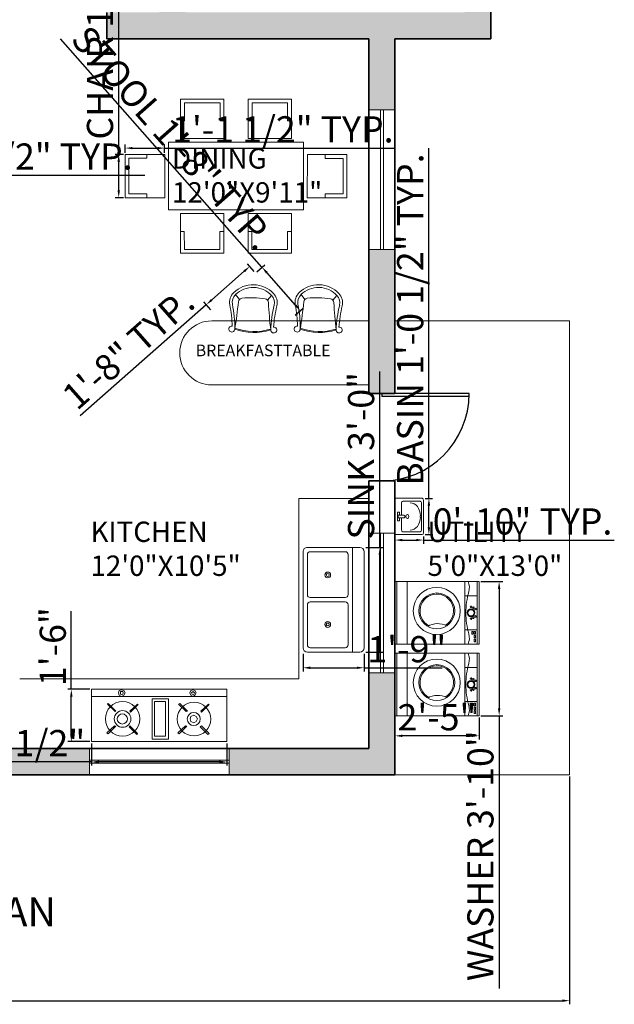
# Model space of a CAD drawing. Units: inches. Extents: x 4606 to 5879, y 1332 to 2209.
# Tile 2 of 7: x 4974 to 5178, y 1332 to 1671. Entities that reach past the tile are written whole.
import ezdxf

# ---------------------------------------------------------------- set-up
doc = ezdxf.new("R2010")
doc.units = ezdxf.units.IN
for name, color, linetype, lineweight in [('A-ANNO-DIMS', 2, 'Continuous', 18), ('A-ANNO-TEXT', 7, 'Continuous', 18), ('A-ANNO-TITL', 7, 'Continuous', 25), ('A-AREA-IDEN', 7, 'Continuous', 18), ('A-DOOR', 4, 'Continuous', 25), ('A-EQPM', 9, 'Continuous', 18), ('A-FLOR-CASE', 32, 'Continuous', 18), ('A-FLOR-PERI', 7, 'Continuous', 20), ('A-FURN', 8, 'Continuous', 18), ('A-WALL', 7, 'Continuous', 35), ('A-WALL-PATT', 252, 'Continuous', 13), ('window', 130, 'Continuous', 18), ('Сантехника', 9, 'Continuous', 18)]:
    doc.layers.add(name, color=color, linetype=linetype, lineweight=lineweight)
doc.styles.get("Standard").update_dxf_attribs({"font": 'arial.ttf'})
doc.dimstyles.new('ISO-25', dxfattribs={"dimtxt": 9, "dimasz": 2.5, "dimexe": 1.25, "dimexo": 0.625, "dimtad": 1, "dimlunit": 3, "dimtxsty": 'Standard', "dimcen": 2.5, "dimadec": 0, "dimazin": 0, "dimtfac": 1, "dimtmove": 0, "dimatfit": 3, "dimfxl": 1, "dimarcsym": 0})

# ---------------------------------------------------------------- blocks, each defined once
blk = doc.blocks.new('D2')
for p, q in [((0, 30), (0, 0)), ((1, 30), (1, 0)), ((0, 0), (1, 0))]:
    blk.add_line(p, q)
blk.add_arc((0, 0), 30, 0, 90)
blk = doc.blocks.new('A$C16EC238A')
for p, q in [((490, 810), (485, 914)), ((148, 493), (45, 507))]:
    blk.add_line(p, q)
for centre, radius, start, end in [((464, 496), 464, 87.0599, 178.502), ((464, 496), 419, 87.0599, 178.502), ((476, 730), 184, 31.9256, 87.0599), ((476, 730), 229, 31.9256, 87.0599), ((2169, 1687), 1760, 209.219, 222.7724), ((2169, 1687), 1715, 209.219, 221.1077), ((1301, -402), 1474, 132.9725, 140.5328), ((1209, -303), 1339, 124.646, 132.9725), ((486, 744), 66, 46.736, 125.0291), ((4628, 5145), 5977, 226.736, 231.1302), ((229, 502), 229, 178.502, 233.6363), ((229, 502), 184, 178.502, 233.6363), ((214, 493), 66, 140.5328, 218.8259), ((62, 930), 910, 293.6787, 331.8832), ((913, 525), 50, 222.7809, 137.6785), ((-856, -1112), 1760, 42.7895, 56.3429), ((-4494, -3296), 5977, 34.4317, 38.8259), ((62, 930), 925, 293.8563, 331.7056), ((-856, -1112), 1715, 44.4541, 56.3429), ((399, 50), 50, 127.8834, 42.7809)]:
    blk.add_arc(centre, radius, start, end)
blk = doc.blocks.new('Sink-double - 36 in top')
for p, q in [((-18, -4), (18, -4)), ((-0.75, -18.5), (-0.75, -6.5)), ((0.75, -6.5), (0.75, -18.5))]:
    blk.add_line(p, q)
for points in [[(-16.5, 0), (16.5, 0)], [(-18, -19.5), (-18, -1.5)], [(18, -1.5), (18, -19.5)], [(-16.5, -18.5), (-16.5, -6.5)], [(-15.5, -5.5), (-1.75, -5.5)], [(1.75, -5.5), (15.5, -5.5)], [(16.5, -6.5), (16.5, -18.5)], [(-1.75, -19.5), (-15.5, -19.5)], [(15.5, -19.5), (1.75, -19.5)], [(16.5, -21), (-16.5, -21)]]:
    blk.add_lwpolyline(points)
for centre, radius in [((-8.5, -12.5), 1), ((-8.5, -12.5), 0.5), ((8.5, -12.5), 1), ((8.5, -12.5), 0.5)]:
    blk.add_circle(centre, radius)
for centre, radius, start, end in [((-16.5, -1.5), 1.5, 90, 180), ((16.5, -1.5), 1.5, 0, 90), ((-15.5, -6.5), 1, 90, 180), ((-1.75, -6.5), 1, 0, 90), ((1.75, -6.5), 1, 90, 180), ((15.5, -6.5), 1, 0, 90), ((-16.5, -19.5), 1.5, 180, 270), ((-15.5, -18.5), 1, 180, 270), ((-1.75, -18.5), 1, 270, 0), ((1.75, -18.5), 1, 180, 270), ((15.5, -18.5), 1, 270, 0), ((16.5, -19.5), 1.5, 270, 0)]:
    blk.add_arc(centre, radius, start, end)
blk = doc.blocks.new('gas 1')
for points in [[(35.93, -1.87), (35.93, 0), (0, 0), (0, -1.87)], [(8.12, -0.94), (8.44, -1.56), (8.91, -1.87), (9.53, -1.56), (9.84, -0.94), (9.53, -0.31), (8.91, -0.16), (8.44, -0.31)], [(8.59, -0.94), (8.75, -1.25), (8.91, -1.41), (9.22, -1.25), (9.37, -0.94), (9.22, -0.78), (8.91, -0.62), (8.75, -0.78)], [(19.84, -13.28), (15.47, -13.28), (15.47, -2.5), (19.84, -2.5)], [(27.03, -0.94), (27.34, -1.56), (27.97, -1.87), (28.59, -1.56), (28.75, -0.94), (28.59, -0.31), (27.97, -0.16), (27.34, -0.31)], [(27.5, -0.94), (27.65, -1.25), (27.97, -1.41), (28.28, -1.25), (28.28, -0.94), (28.28, -0.62), (27.97, -0.62), (27.65, -0.62)], [(4.84, -3.91), (4.69, -4.06), (6.72, -6.09), (6.87, -5.78)], [(12.81, -3.91), (12.5, -3.75), (10.47, -5.78), (10.78, -5.94)], [(19.22, -12.5), (16.25, -12.5), (16.25, -3.28), (19.22, -3.28)], [(23.75, -3.91), (23.59, -4.06), (25.62, -6.09), (25.78, -5.78)], [(31.71, -3.91), (31.56, -3.75), (29.53, -5.78), (29.68, -5.94)], [(7.81, -7.81), (8.12, -8.59), (8.75, -8.91), (9.53, -8.59), (9.69, -7.81), (9.53, -7.19), (8.75, -6.87), (8.12, -7.19)], [(7.03, -10), (6.72, -9.69), (4.69, -11.72), (5, -12.03)], [(12.97, -11.56), (10.94, -9.69), (10.62, -9.84), (12.65, -11.87)], [(23.75, -11.72), (23.9, -12.03), (25.93, -10), (25.78, -9.69)], [(31.87, -11.56), (29.84, -9.69), (29.53, -9.84), (31.56, -11.87)]]:
    blk.add_lwpolyline(points, close=True)
blk.add_lwpolyline([(35.93, -1.87), (35.93, -13.9), (0, -13.9), (0, -1.87)])
for centre, radius in [((8.7, -7.92), 4.48), ((27.7, -7.86), 4.58), ((8.77, -7.89), 1.74), ((27.69, -7.89), 2.22), ((27.76, -7.89), 1.35)]:
    blk.add_circle(centre, radius)
blk = doc.blocks.new('wash')
at = {"layer": 'Сантехника'}
for p, q in [((4817.13, 2840.92), (4788.24, 2840.92)), ((4788.24, 2819.46), (4788.24, 2840.92)), ((4788.93, 2819.46), (4788.93, 2840.92)), ((4793.08, 2819.46), (4793.08, 2840.92)), ((4812.98, 2819.46), (4812.98, 2840.92)), ((4816.44, 2819.46), (4816.44, 2840.92)), ((4817.13, 2819.46), (4817.13, 2840.92)), ((4793.08, 2836.07), (4788.93, 2836.07)), ((4793.08, 2824.31), (4788.93, 2824.31)), ((4817.13, 2819.46), (4788.24, 2819.46)), ((4817.13, 2816.27), (4788.24, 2816.27)), ((4788.24, 2794.82), (4788.24, 2816.27)), ((4788.93, 2794.82), (4788.93, 2816.27)), ((4793.08, 2794.82), (4793.08, 2816.27)), ((4812.98, 2794.82), (4812.98, 2816.27)), ((4816.44, 2794.82), (4816.44, 2816.27)), ((4817.13, 2794.82), (4817.13, 2816.27)), ((4793.08, 2811.43), (4788.93, 2811.43)), ((4793.08, 2799.66), (4788.93, 2799.66)), ((4817.13, 2794.82), (4788.24, 2794.82))]:
    blk.add_line(p, q, dxfattribs=at)
for points in [[(4789.4, 2839.27), (4789.4, 2840.17), (4789.9, 2840.17), (4789.9, 2839.27)], [(4789.4, 2837.95), (4789.4, 2838.85), (4789.9, 2838.85), (4789.9, 2837.95)], [(4789.4, 2836.64), (4789.4, 2837.53), (4789.9, 2837.53), (4789.9, 2836.64)], [(4790.27, 2836.64), (4790.27, 2837.53), (4790.77, 2837.53), (4790.77, 2836.64)], [(4789.4, 2814.62), (4789.4, 2815.52), (4789.9, 2815.52), (4789.9, 2814.62)], [(4789.4, 2813.31), (4789.4, 2814.2), (4789.9, 2814.2), (4789.9, 2813.31)], [(4789.4, 2811.99), (4789.4, 2812.89), (4789.9, 2812.89), (4789.9, 2811.99)], [(4790.27, 2811.99), (4790.27, 2812.89), (4790.77, 2812.89), (4790.77, 2811.99)]]:
    blk.add_lwpolyline(points, close=True, dxfattribs=at)
for centre, radius in [((4802.77, 2829.54), 8.1), ((4802.77, 2829.54), 6.17), ((4789.46, 2831.45), 0.271), ((4790.98, 2830.19), 1.34), ((4790.19, 2831.93), 0.271), ((4790.98, 2830.19), 1.07), ((4790.98, 2832.18), 0.271), ((4789.46, 2828.92), 0.271), ((4790.19, 2828.4), 0.271), ((4790.98, 2828.15), 0.271), ((4802.77, 2804.9), 8.1), ((4802.77, 2804.9), 6.17), ((4789.46, 2806.8), 0.271), ((4790.98, 2805.55), 1.34), ((4790.19, 2807.28), 0.271), ((4790.98, 2805.55), 1.07), ((4790.98, 2807.53), 0.271), ((4789.46, 2804.27), 0.271), ((4790.19, 2803.75), 0.271), ((4790.98, 2803.5), 0.271)]:
    blk.add_circle(centre, radius, dxfattribs=at)
for centre, radius, start, end in [((4796.44, 2838.85), 4.89, 154.895, 196.6068), ((4762.87, 2829.66), 29.92, 1.0206, 15.0937), ((4802.77, 2829.54), 5.77, 121.8067, 62.1506), ((4802.39, 2840.74), 6.83, 243.19, 300.7673), ((4762.87, 2830.72), 29.92, 344.9063, 358.9794), ((4796.44, 2821.54), 4.89, 163.3932, 205.105), ((4796.44, 2814.2), 4.89, 154.895, 196.6068), ((4762.87, 2805.01), 29.92, 1.0206, 15.0937), ((4802.77, 2804.9), 5.77, 121.8067, 62.1506), ((4802.39, 2816.1), 6.83, 243.19, 300.7673), ((4762.87, 2806.08), 29.92, 344.9063, 358.9794), ((4796.44, 2796.89), 4.89, 163.3932, 205.105)]:
    blk.add_arc(centre, radius, start, end, dxfattribs=at)
blk = doc.blocks.new('Rac7')
at = {"color": 0}
for p, q in [((-39501, -24232), (-39501, -23830)), ((-39474, -23808), (-38988, -23808)), ((-39457, -23859), (-39457, -24115)), ((-39032, -23838), (-39430, -23838)), ((-39221, -23855), (-39241, -23855)), ((-39005, -24115), (-39005, -23859)), ((-39005, -23859), (-39005, -23859)), ((-38961, -23830), (-38961, -24232)), ((-39430, -24136), (-39253, -24136)), ((-39297, -24164), (-39253, -24164)), ((-39297, -24194), (-39297, -24164)), ((-39253, -24186), (-39253, -24094)), ((-39209, -24186), (-39209, -24094)), ((-39209, -24136), (-39032, -24136)), ((-39209, -24164), (-39165, -24164)), ((-39165, -24164), (-39165, -24194)), ((-38961, -24232), (-39501, -24232)), ((-39165, -24194), (-39297, -24194)), ((-39253, -24186), (-39209, -24186))]:
    blk.add_line(p, q, dxfattribs=at)
at = {"color": 0, "extrusion": (0, 0, -1)}
for centre, major_axis, start_param, end_param in [((-39474, -23830), (-27, 0), 0, 1.570796), ((-39430, -23859), (-27, 0), 0, 1.570796), ((-39241, -24007), (-194, 0), 0, 1.570796), ((-39221, -24007), (-194, 0), 1.570796, 3.141593), ((-39032, -23859), (-27, 0), 1.570796, 3.141593), ((-38988, -23830), (-27, 0), 1.570796, 3.141593), ((-39430, -24115), (-27, 0), -1.570796, 0), ((-39231, -24104), (-25.3, 0), 0.552816, 2.588777), ((-39032, -24115), (-27, 0), -3.141593, -1.570796)]:
    blk.add_ellipse(centre, major_axis=major_axis, ratio=0.785714, start_param=start_param, end_param=end_param, dxfattribs=at)
blk.add_ellipse((-39231, -24048), major_axis=(-27.9, 0), ratio=0.785714, dxfattribs=at)
blk = doc.blocks.new('GLAZING-48IN')
for p, q in [((0, 0), (0, 48)), ((1, 0), (1, 48))]:
    blk.add_line(p, q)
blk = doc.blocks.new('DINING-CHAIR')
for p, q in [((0, 14.84), (13.57, 14.84)), ((0, 0), (0, 14.84)), ((1.28, 13.56), (7.42, 13.56)), ((1.28, 1.32), (1.28, 13.56)), ((7.42, 13.56), (7.42, 14.84)), ((13.57, 0), (13.57, 14.84)), ((0, 0), (13.57, 0)), ((7.42, 1.32), (1.28, 1.32)), ((7.42, 0), (7.42, 1.32))]:
    blk.add_line(p, q)
blk = doc.blocks.new('*D83')
at = {"layer": 'A-ANNO-DIMS', "color": 0, "lineweight": -2, "transparency": 16777216}
for p, q in [((5007.89, 1624.4), (5007.89, 1725.52)), ((5009.49, 1624.4), (5006.64, 1624.4)), ((5007.89, 1612.06), (5007.89, 1621.9)), ((5009.49, 1609.56), (5006.64, 1609.56))]:
    blk.add_line(p, q, dxfattribs=at)
at = {"layer": 'A-ANNO-DIMS', "color": 0, "transparency": 16777216}
for points in [[(5007.47, 1621.9), (5008.31, 1621.9), (5007.89, 1624.4)], [(5007.47, 1612.06), (5008.31, 1612.06), (5007.89, 1609.56)]]:
    blk.add_solid(points, dxfattribs=at)
at = {"layer": 'Defpoints', "color": 0, "transparency": 16777216}
for p in [(5007.89, 1624.4), (5010.11, 1624.4), (5010.11, 1609.56)]:
    blk.add_point(p, dxfattribs=at)
at = {"layer": 'A-ANNO-DIMS', "color": 0, "transparency": 16777216, "insert": (5002.61, 1676.21), "char_height": 9, "attachment_point": 5, "rotation": 90}
blk.add_mtext('CHAIR 1\'-3" TYP.', dxfattribs=at)
blk = doc.blocks.new('*D84')
at = {"layer": 'A-ANNO-DIMS', "color": 0, "lineweight": -2, "transparency": 16777216}
for p, q in [((5010.11, 1625.03), (5010.11, 1627.88)), ((5012.61, 1626.63), (5021.18, 1626.63)), ((5023.68, 1625.03), (5023.68, 1627.88)), ((5023.68, 1626.63), (5102.42, 1626.63))]:
    blk.add_line(p, q, dxfattribs=at)
at = {"layer": 'A-ANNO-DIMS', "color": 0, "transparency": 16777216}
for points in [[(5012.61, 1627.04), (5012.61, 1626.21), (5010.11, 1626.63)], [(5021.18, 1627.04), (5021.18, 1626.21), (5023.68, 1626.63)]]:
    blk.add_solid(points, dxfattribs=at)
at = {"layer": 'Defpoints', "color": 0, "transparency": 16777216}
for p in [(5023.68, 1626.63), (5010.11, 1624.4), (5023.68, 1624.4)]:
    blk.add_point(p, dxfattribs=at)
at = {"layer": 'A-ANNO-DIMS', "color": 0, "transparency": 16777216, "insert": (5064.3, 1631.91), "char_height": 9, "attachment_point": 5}
blk.add_mtext('1\'-1 1/2" TYP.', dxfattribs=at)
blk = doc.blocks.new('*D85')
at = {"layer": 'A-ANNO-DIMS', "color": 0, "lineweight": -2, "transparency": 16777216}
for p, q in [((5114.51, 1506.24), (5114.51, 1626.65)), ((5113.27, 1506.24), (5115.76, 1506.24)), ((5114.51, 1496.28), (5114.51, 1503.74)), ((5113.27, 1493.78), (5115.76, 1493.78))]:
    blk.add_line(p, q, dxfattribs=at)
at = {"layer": 'A-ANNO-DIMS', "color": 0, "transparency": 16777216}
for points in [[(5114.09, 1503.74), (5114.93, 1503.74), (5114.51, 1506.24)], [(5114.09, 1496.28), (5114.93, 1496.28), (5114.51, 1493.78)]]:
    blk.add_solid(points, dxfattribs=at)
at = {"layer": 'Defpoints', "color": 0, "transparency": 16777216}
for p in [(5112.64, 1506.24), (5114.51, 1506.24), (5112.64, 1493.78)]:
    blk.add_point(p, dxfattribs=at)
at = {"layer": 'A-ANNO-DIMS', "color": 0, "transparency": 16777216, "insert": (5109.23, 1567.69), "char_height": 9, "attachment_point": 5, "rotation": 90}
blk.add_mtext('BASIN 1\'-0 1/2" TYP.', dxfattribs=at)
blk = doc.blocks.new('*D86')
at = {"layer": 'A-ANNO-DIMS', "color": 0, "lineweight": -2, "transparency": 16777216}
for p, q in [((5102.85, 1493.15), (5102.85, 1490.66)), ((5112.64, 1493.15), (5112.64, 1490.66)), ((5105.35, 1491.91), (5110.14, 1491.91)), ((5112.64, 1491.91), (5178.24, 1491.91))]:
    blk.add_line(p, q, dxfattribs=at)
at = {"layer": 'A-ANNO-DIMS', "color": 0, "transparency": 16777216}
for points in [[(5105.35, 1492.32), (5105.35, 1491.49), (5102.85, 1491.91)], [(5110.14, 1492.32), (5110.14, 1491.49), (5112.64, 1491.91)]]:
    blk.add_solid(points, dxfattribs=at)
at = {"layer": 'Defpoints', "color": 0, "transparency": 16777216}
for p in [(5102.85, 1493.78), (5112.64, 1493.78), (5112.64, 1491.91)]:
    blk.add_point(p, dxfattribs=at)
at = {"layer": 'A-ANNO-DIMS', "color": 0, "transparency": 16777216, "insert": (5146.69, 1497.13), "char_height": 9, "attachment_point": 5}
blk.add_mtext('0\'-10" TYP.', dxfattribs=at)
blk = doc.blocks.new('*D87')
at = {"layer": 'A-ANNO-DIMS', "color": 0, "lineweight": -2, "transparency": 16777216}
for p, q in [((4826.48, 1622.61), (4826.48, 1616.03)), ((4866.23, 1622.61), (4866.23, 1616.03)), ((4828.98, 1617.28), (4863.73, 1617.28)), ((4866.23, 1617.28), (5016.88, 1617.28))]:
    blk.add_line(p, q, dxfattribs=at)
at = {"layer": 'A-ANNO-DIMS', "color": 0, "transparency": 16777216}
for points in [[(4828.98, 1617.69), (4828.98, 1616.86), (4826.48, 1617.28)], [(4863.73, 1617.69), (4863.73, 1616.86), (4866.23, 1617.28)]]:
    blk.add_solid(points, dxfattribs=at)
at = {"layer": 'Defpoints', "color": 0, "transparency": 16777216}
for p in [(4826.48, 1623.24), (4866.23, 1623.24), (4866.23, 1617.28)]:
    blk.add_point(p, dxfattribs=at)
at = {"layer": 'A-ANNO-DIMS', "color": 0, "transparency": 16777216, "insert": (4942.8, 1622.56), "char_height": 9, "attachment_point": 5}
blk.add_mtext('ARMCHAIR 3\'-3 1/2" TYP.', dxfattribs=at)
blk = doc.blocks.new('*D101')
at = {"layer": 'A-ANNO-DIMS', "color": 0, "lineweight": -2, "transparency": 16777216}
for p, q in [((5057.14, 1585.7), (4987.91, 1664.21)), ((5055.37, 1584.13), (5058.08, 1586.52)), ((5068.67, 1572.62), (5058.79, 1583.82)), ((5068.55, 1569.18), (5071.26, 1571.57))]:
    blk.add_line(p, q, dxfattribs=at)
at = {"layer": 'A-ANNO-DIMS', "color": 0, "transparency": 16777216}
for points in [[(5059.11, 1584.1), (5058.48, 1583.55), (5057.14, 1585.7)], [(5068.98, 1572.9), (5068.36, 1572.35), (5070.32, 1570.75)]]:
    blk.add_solid(points, dxfattribs=at)
at = {"layer": 'Defpoints', "color": 0, "transparency": 16777216}
for p in [(5057.14, 1585.7), (5054.9, 1583.72), (5068.08, 1568.77)]:
    blk.add_point(p, dxfattribs=at)
at = {"layer": 'A-ANNO-DIMS', "color": 0, "transparency": 16777216, "insert": (5025.66, 1629.38), "char_height": 9, "attachment_point": 5, "rotation": 311.4042}
blk.add_mtext('STOOL 1\'-8" TYP.', dxfattribs=at)
blk = doc.blocks.new('*D102')
at = {"layer": 'A-ANNO-DIMS', "color": 0, "lineweight": -2, "transparency": 16777216}
for p, q in [((5051.05, 1584.31), (5039.88, 1574.46)), ((5054.49, 1584.19), (5052.1, 1586.9)), ((5039.56, 1571.03), (5037.17, 1573.74)), ((5038, 1572.81), (4994.68, 1534.6))]:
    blk.add_line(p, q, dxfattribs=at)
at = {"layer": 'A-ANNO-DIMS', "color": 0, "transparency": 16777216}
for points in [[(5050.77, 1584.62), (5051.32, 1584), (5052.92, 1585.96)], [(5039.6, 1574.77), (5040.15, 1574.15), (5038, 1572.81)]]:
    blk.add_solid(points, dxfattribs=at)
at = {"layer": 'Defpoints', "color": 0, "transparency": 16777216}
for p in [(5054.9, 1583.72), (5038, 1572.81), (5039.98, 1570.56)]:
    blk.add_point(p, dxfattribs=at)
at = {"layer": 'A-ANNO-DIMS', "color": 0, "transparency": 16777216, "insert": (5011.95, 1556.79), "char_height": 9, "attachment_point": 5, "rotation": 41.4042}
blk.add_mtext('1\'-8" TYP.', dxfattribs=at)
blk = doc.blocks.new('*D107')
at = {"layer": 'A-ANNO-DIMS', "color": 0, "lineweight": -2, "transparency": 16777216}
for p, q in [((5097.64, 1489.4), (5097.64, 1549.87)), ((5092.87, 1489.4), (5098.89, 1489.4)), ((5097.64, 1455.9), (5097.64, 1486.9)), ((5092.87, 1453.4), (5098.89, 1453.4))]:
    blk.add_line(p, q, dxfattribs=at)
at = {"layer": 'A-ANNO-DIMS', "color": 0, "transparency": 16777216}
for points in [[(5097.23, 1486.9), (5098.06, 1486.9), (5097.64, 1489.4)], [(5097.23, 1455.9), (5098.06, 1455.9), (5097.64, 1453.4)]]:
    blk.add_solid(points, dxfattribs=at)
at = {"layer": 'Defpoints', "color": 0, "transparency": 16777216}
for p in [(5092.24, 1489.4), (5097.64, 1489.4), (5092.24, 1453.4)]:
    blk.add_point(p, dxfattribs=at)
at = {"layer": 'A-ANNO-DIMS', "color": 0, "transparency": 16777216, "insert": (5092.36, 1520.89), "char_height": 9, "attachment_point": 5, "rotation": 90}
blk.add_mtext('SINK 3\'-0"', dxfattribs=at)
blk = doc.blocks.new('*D108')
at = {"layer": 'A-ANNO-DIMS', "color": 0, "lineweight": -2, "transparency": 16777216}
for p, q in [((5071.24, 1452.78), (5071.24, 1446.75)), ((5092.24, 1452.78), (5092.24, 1446.75)), ((5073.74, 1448), (5089.74, 1448)), ((5092.24, 1448), (5119.07, 1448))]:
    blk.add_line(p, q, dxfattribs=at)
at = {"layer": 'A-ANNO-DIMS', "color": 0, "transparency": 16777216}
for points in [[(5073.74, 1448.42), (5073.74, 1447.59), (5071.24, 1448)], [(5089.74, 1448.42), (5089.74, 1447.59), (5092.24, 1448)]]:
    blk.add_solid(points, dxfattribs=at)
at = {"layer": 'Defpoints', "color": 0, "transparency": 16777216}
for p in [(5071.24, 1453.4), (5092.24, 1453.4), (5092.24, 1448)]:
    blk.add_point(p, dxfattribs=at)
at = {"layer": 'A-ANNO-DIMS', "color": 0, "transparency": 16777216, "insert": (5106.91, 1453.22), "char_height": 9, "attachment_point": 5}
blk.add_mtext('1\'-9"', dxfattribs=at)
blk = doc.blocks.new('*D109')
at = {"layer": 'A-ANNO-DIMS', "color": 0, "lineweight": -2, "transparency": 16777216}
for p, q in [((4998.57, 1422), (4998.57, 1414.41)), ((5045.02, 1422), (5045.02, 1414.41)), ((4998.57, 1415.66), (4912.68, 1415.66)), ((5042.52, 1415.66), (5001.07, 1415.66))]:
    blk.add_line(p, q, dxfattribs=at)
at = {"layer": 'A-ANNO-DIMS', "color": 0, "transparency": 16777216}
for points in [[(5001.07, 1416.08), (5001.07, 1415.25), (4998.57, 1415.66)], [(5042.52, 1416.08), (5042.52, 1415.25), (5045.02, 1415.66)]]:
    blk.add_solid(points, dxfattribs=at)
at = {"layer": 'Defpoints', "color": 0, "transparency": 16777216}
for p in [(4998.57, 1422.63), (5045.02, 1422.63), (4998.57, 1415.66)]:
    blk.add_point(p, dxfattribs=at)
at = {"layer": 'A-ANNO-DIMS', "color": 0, "transparency": 16777216, "insert": (4954.38, 1420.95), "char_height": 9, "attachment_point": 5}
blk.add_mtext('HOB 3\'-10 1/2"', dxfattribs=at)
blk = doc.blocks.new('*D110')
at = {"layer": 'A-ANNO-DIMS', "color": 0, "lineweight": -2, "transparency": 16777216}
for p, q in [((4991.6, 1440.6), (4991.6, 1467.43)), ((4997.95, 1440.6), (4990.35, 1440.6)), ((4991.6, 1425.13), (4991.6, 1438.1)), ((4997.95, 1422.63), (4990.35, 1422.63))]:
    blk.add_line(p, q, dxfattribs=at)
at = {"layer": 'A-ANNO-DIMS', "color": 0, "transparency": 16777216}
for points in [[(4991.19, 1438.1), (4992.02, 1438.1), (4991.6, 1440.6)], [(4991.19, 1425.13), (4992.02, 1425.13), (4991.6, 1422.63)]]:
    blk.add_solid(points, dxfattribs=at)
at = {"layer": 'Defpoints', "color": 0, "transparency": 16777216}
for p in [(4991.6, 1440.6), (4998.57, 1440.6), (4998.57, 1422.63)]:
    blk.add_point(p, dxfattribs=at)
at = {"layer": 'A-ANNO-DIMS', "color": 0, "transparency": 16777216, "insert": (4986.38, 1455.27), "char_height": 9, "attachment_point": 5, "rotation": 90}
blk.add_mtext('1\'-6"', dxfattribs=at)
blk = doc.blocks.new('*D111')
at = {"layer": 'A-ANNO-DIMS', "color": 0, "lineweight": -2, "transparency": 16777216}
for p, q in [((5132.37, 1477.63), (5139.91, 1477.63)), ((5138.66, 1475.13), (5138.66, 1434.03)), ((5132.37, 1431.53), (5139.91, 1431.53)), ((5138.66, 1431.53), (5138.66, 1337.81))]:
    blk.add_line(p, q, dxfattribs=at)
at = {"layer": 'A-ANNO-DIMS', "color": 0, "transparency": 16777216}
for points in [[(5138.24, 1475.13), (5139.08, 1475.13), (5138.66, 1477.63)], [(5138.24, 1434.03), (5139.08, 1434.03), (5138.66, 1431.53)]]:
    blk.add_solid(points, dxfattribs=at)
at = {"layer": 'Defpoints', "color": 0, "transparency": 16777216}
for p in [(5131.74, 1477.63), (5131.74, 1431.53), (5138.66, 1431.53)]:
    blk.add_point(p, dxfattribs=at)
at = {"layer": 'A-ANNO-DIMS', "color": 0, "transparency": 16777216, "insert": (5133.38, 1383.42), "char_height": 9, "attachment_point": 5, "rotation": 90}
blk.add_mtext('WASHER 3\'-10"', dxfattribs=at)
blk = doc.blocks.new('*D112')
at = {"layer": 'A-ANNO-DIMS', "color": 0, "lineweight": -2, "transparency": 16777216}
for p, q in [((5102.85, 1430.9), (5102.85, 1423.36)), ((5131.74, 1430.9), (5131.74, 1423.36)), ((5129.24, 1424.61), (5105.35, 1424.61))]:
    blk.add_line(p, q, dxfattribs=at)
at = {"layer": 'A-ANNO-DIMS', "color": 0, "transparency": 16777216}
for points in [[(5105.35, 1425.03), (5105.35, 1424.2), (5102.85, 1424.61)], [(5129.24, 1425.03), (5129.24, 1424.2), (5131.74, 1424.61)]]:
    blk.add_solid(points, dxfattribs=at)
at = {"layer": 'Defpoints', "color": 0, "transparency": 16777216}
for p in [(5102.85, 1431.53), (5131.74, 1431.53), (5102.85, 1424.61)]:
    blk.add_point(p, dxfattribs=at)
at = {"layer": 'A-ANNO-DIMS', "color": 0, "transparency": 16777216, "insert": (5117.3, 1429.83), "char_height": 9, "attachment_point": 5}
blk.add_mtext('2\'-5"', dxfattribs=at)
blk = doc.blocks.new('*D113')
at = {"layer": 'A-ANNO-DIMS', "color": 0, "lineweight": -2, "transparency": 16777216}
for p, q in [((4658.85, 1410.61), (4658.85, 1332.33)), ((5162.85, 1410.61), (5162.85, 1332.33)), ((4661.35, 1333.58), (5160.35, 1333.58))]:
    blk.add_line(p, q, dxfattribs=at)
at = {"layer": 'A-ANNO-DIMS', "color": 0, "transparency": 16777216}
for points in [[(4661.35, 1334), (4661.35, 1333.16), (4658.85, 1333.58)], [(5160.35, 1334), (5160.35, 1333.16), (5162.85, 1333.58)]]:
    blk.add_solid(points, dxfattribs=at)
at = {"layer": 'Defpoints', "color": 0, "transparency": 16777216}
for p in [(4658.85, 1411.24), (5162.85, 1411.24), (5162.85, 1333.58)]:
    blk.add_point(p, dxfattribs=at)
at = {"layer": 'A-ANNO-DIMS', "color": 0, "transparency": 16777216, "insert": (4910.85, 1338.8), "char_height": 9, "attachment_point": 5}
blk.add_mtext('42\'-0"', dxfattribs=at)

msp = doc.modelspace()

# ---------------------------------------------------------------- hatches: boundary and pattern name
at = {"layer": 'A-WALL-PATT', "transparency": 33554687}
h = msp.add_hatch(color=256, dxfattribs=at)
h.dxf.hatch_style = 1
h.paths.add_polyline_path([(4715.85, 2081.239), (4658.85, 2081.239), (4658.85, 2054.239), (4667.85, 2054.239), (4667.85, 2072.239), (4715.85, 2072.239)])
h.paths.add_polyline_path([(4868.85, 2081.239), (4787.85, 2081.239), (4787.85, 2072.239), (4835.85, 2072.239), (4835.85, 1955.239), (4844.85, 1955.239), (4844.85, 1970.239), (4850.85, 1970.239), (4850.85, 1976.239), (4844.85, 1976.239), (4844.85, 2072.239), (4868.85, 2072.239)])
h.paths.add_polyline_path([(4940.85, 2081.239), (4892.85, 2081.239), (4892.85, 2072.239), (4916.85, 2072.239), (4916.85, 1976.239), (4880.85, 1976.239), (4880.85, 1970.239), (4916.85, 1970.239), (4916.85, 1904.239), (4844.85, 1904.239), (4844.85, 1925.239), (4835.85, 1925.239), (4835.85, 1904.239), (4832.85, 1904.239), (4832.85, 1895.239), (4919.85, 1895.239), (4991.85, 1895.239), (4991.85, 1904.239), (4988.85, 1904.239), (4988.85, 1925.239), (4982.85, 1925.239), (4982.85, 1904.239), (4922.85, 1904.239), (4922.85, 1970.239), (4946.85, 1970.239), (4946.85, 1976.239), (4922.85, 1976.239), (4922.85, 2072.239), (4940.85, 2072.239)])
h.paths.add_polyline_path([(5021.85, 2081.239), (4964.85, 2081.239), (4964.85, 2072.239), (4982.85, 2072.239), (4982.85, 1976.239), (4976.85, 1976.239), (4976.85, 1970.239), (4982.85, 1970.239), (4982.85, 1955.239), (4988.85, 1955.239), (4988.85, 2072.239), (5021.85, 2072.239)])
h.paths.add_polyline_path([(5135.85, 2081.239), (5093.85, 2081.239), (5093.85, 2072.239), (5126.85, 2072.239), (5126.85, 2054.239), (5135.85, 2054.239)])
h.paths.add_polyline_path([(5135.85, 2006.239), (5126.85, 2006.239), (5126.85, 1976.239), (5135.85, 1976.239)])
h.paths.add_polyline_path([(5135.85, 1928.239), (5126.85, 1928.239), (5126.85, 1904.239), (5027.85, 1904.239), (5027.85, 1895.239), (5126.85, 1895.239), (5126.85, 1871.239), (5135.85, 1871.239)])
h.paths.add_polyline_path([(4796.85, 1904.239), (4667.85, 1904.239), (4667.85, 1922.239), (4658.85, 1922.239), (4658.85, 1895.239), (4766.85, 1895.239), (4766.85, 1674.239), (4775.85, 1674.239), (4775.85, 1895.239), (4796.85, 1895.239)])
h.paths.add_polyline_path([(4667.85, 2006.239), (4658.85, 2006.239), (4658.85, 1970.239), (4667.85, 1970.239)])
h.paths.add_polyline_path([(4880.85, 1545.239), (4940.85, 1545.239), (4940.85, 1542.239), (4949.85, 1542.239), (4949.85, 1566.239), (4940.85, 1566.239), (4940.85, 1554.239), (4880.85, 1554.239), (4880.85, 1614.239), (4940.85, 1614.239), (4940.85, 1602.239), (4949.85, 1602.239), (4949.85, 1623.239), (4866.739, 1623.239), (4826.85, 1623.239), (4826.85, 1614.239), (4871.85, 1614.239), (4871.85, 1554.239), (4826.85, 1554.239), (4826.85, 1545.239), (4871.85, 1545.239), (4871.85, 1411.239), (4997.85, 1411.239), (4997.85, 1420.239), (4949.85, 1420.239), (4949.85, 1512.239), (4940.85, 1512.239), (4940.85, 1420.239), (4880.85, 1420.239)])
h.paths.add_polyline_path([(5102.85, 1446.239), (5093.85, 1446.239), (5093.85, 1420.239), (5045.85, 1420.239), (5045.85, 1411.239), (5102.85, 1411.239)])
h.paths.add_polyline_path([(5102.85, 1591.739), (5093.85, 1591.739), (5093.85, 1542.239), (5102.85, 1542.239)])
h.paths.add_polyline_path([(5135.85, 1691.239), (5126.85, 1691.239), (5126.85, 1673.239), (5030.85, 1673.239), (5030.85, 1676.239), (5021.85, 1676.239), (5021.85, 1673.239), (5003.85, 1673.239), (5003.85, 1664.239), (5093.85, 1664.239), (5093.85, 1639.739), (5102.85, 1639.739), (5102.85, 1664.239), (5135.85, 1664.239)])
h.paths.add_polyline_path([(5135.85, 1823.239), (5126.85, 1823.239), (5126.85, 1799.239), (5028.85, 1799.239), (5028.85, 1790.239), (5057.85, 1790.239), (5057.85, 1784.239), (5066.85, 1784.239), (5066.85, 1790.239), (5126.85, 1790.239), (5126.85, 1742.239), (5066.85, 1742.239), (5066.85, 1748.239), (5057.85, 1748.239), (5057.85, 1742.239), (5021.85, 1742.239), (5021.85, 1706.239), (5030.85, 1706.239), (5030.85, 1733.239), (5126.85, 1733.239), (5126.85, 1715.239), (5135.85, 1715.239)])
h.paths.add_polyline_path([(4775.85, 1602.239), (4766.85, 1602.239), (4766.85, 1474.239), (4775.85, 1474.239), (4775.85, 1545.239), (4778.85, 1545.239), (4778.85, 1554.239), (4775.85, 1554.239)])
h.paths.add_polyline_path([(4692.58, 1635.003), (4749.356, 1635.003), (4749.356, 1665.418), (4692.58, 1665.418)], flags=9)

# ---------------------------------------------------------------- linework, layer by layer
at = {"layer": 'A-FLOR-CASE'}
for p, q in [((5093.85, 1567.239), (5039.85, 1567.239)), ((5039.85, 1545.239), (5093.85, 1545.239)), ((5069.85, 1506.239), (5093.85, 1506.239)), ((5069.85, 1506.239), (5069.85, 1444.239)), ((4973.85, 1444.239), (5069.85, 1444.239))]:
    msp.add_line(p, q, dxfattribs=at)
msp.add_arc((5039.85, 1556.239), 11, 90, 270, dxfattribs=at)
at = {"layer": 'A-FLOR-PERI'}
for p, q in [((5162.85, 1567.239), (5102.85, 1567.239)), ((5162.85, 1411.239), (5162.85, 1567.239)), ((5102.85, 1411.239), (5162.85, 1411.239))]:
    msp.add_line(p, q, dxfattribs=at)
at = {"layer": 'A-FURN'}
for p, q in [((5024.96, 1628.634), (5071.437, 1628.634)), ((5024.96, 1605.372), (5024.96, 1628.634)), ((5071.437, 1628.634), (5071.437, 1605.372)), ((5071.437, 1605.372), (5024.96, 1605.372))]:
    msp.add_line(p, q, dxfattribs=at)
at = {"layer": 'A-WALL'}
for p, q in [((5003.85, 1664.239), (5003.85, 1673.239)), ((5093.85, 1664.239), (5003.85, 1664.239)), ((5093.85, 1664.239), (5093.85, 1542.239)), ((5135.85, 1664.239), (5102.85, 1664.239)), ((5102.85, 1664.239), (5102.85, 1542.239)), ((5093.85, 1542.239), (5102.85, 1542.239)), ((5093.85, 1512.239), (5093.85, 1420.239)), ((5093.85, 1512.239), (5102.85, 1512.239)), ((5102.85, 1512.239), (5102.85, 1411.239)), ((4949.85, 1420.239), (5093.85, 1420.239))]:
    msp.add_line(p, q, dxfattribs=at)
msp.add_lwpolyline([(5135.85, 1664.239), (5135.85, 2081.239), (4658.85, 2081.239), (4658.85, 1411.239), (5102.85, 1411.239)], dxfattribs=at)
at = {"layer": 'window'}
for p, q in [((5093.85, 1639.739), (5102.85, 1639.739)), ((5093.85, 1591.739), (5102.85, 1591.739)), ((5093.85, 1494.239), (5102.85, 1494.239)), ((5093.85, 1446.239), (5102.85, 1446.239)), ((4997.85, 1420.239), (4997.85, 1411.239)), ((5045.85, 1420.239), (5045.85, 1411.239))]:
    msp.add_line(p, q, dxfattribs=at)

# ---------------------------------------------------------------- block references
at = {"layer": 'A-DOOR', "rotation": 270}
msp.add_blockref('D2', (5098.35, 1542.239), dxfattribs=at)
at = {"layer": 'A-EQPM', "rotation": 180}
msp.add_blockref('wash', (9919.983, 4272.446), dxfattribs=at)
at = {"layer": 'A-EQPM', "xscale": -1.292580420916565, "yscale": 1.292580420916565, "zscale": 1.292580420916565}
msp.add_blockref('gas 1', (5045.017, 1440.602), dxfattribs=at)
at = {"layer": 'A-FURN'}
for p, rotation in [((5029.155, 1643.474), 269.929330337337), ((5052.4, 1643.467), 269.9790238270808), ((5086.294, 1624.413), 179.9314884092734), ((5044.007, 1590.537), 90.03023468100444), ((5067.255, 1590.534), 90.01148952389279)]:
    msp.add_blockref('DINING-CHAIR', p, dxfattribs=dict(at, rotation=rotation))
msp.add_blockref('DINING-CHAIR', (5010.115, 1609.564), dxfattribs=at)
at = {"layer": 'A-FURN', "xscale": -0.020608905712957, "yscale": 0.020608905712957, "zscale": 0.020608905712957, "rotation": 41.40420178219905}
for p in [(5068.029, 1568.768), (5090.511, 1568.768)]:
    msp.add_blockref('A$C16EC238A', p, dxfattribs=at)
at = {"layer": 'window'}
for p in [(5097.85, 1591.739), (5097.85, 1446.239)]:
    msp.add_blockref('GLAZING-48IN', p, dxfattribs=at)
at = {"layer": 'window', "rotation": 270.0000000000001}
msp.add_blockref('GLAZING-48IN', (4997.85, 1416.239), dxfattribs=at)
at = {"layer": 'Сантехника', "xscale": -0.0231094998546128, "yscale": 0.0231094998546128, "zscale": 0.0231094998546128, "rotation": 270}
msp.add_blockref('Rac7', (5662.842, 2406.616), dxfattribs=at)
at = {"layer": 'Сантехника', "xscale": -1, "rotation": 270}
msp.add_blockref('Sink-double - 36 in top', (5092.244, 1471.402), dxfattribs=at)

# ---------------------------------------------------------------- texts
at = {"layer": 'A-ANNO-TEXT', "insert": (5034.364, 1559.08), "char_height": 4, "attachment_point": 1}
msp.add_mtext_dynamic_manual_height_columns('{\\fTimes New Roman|b0|i0|c0|p18;BREAKFASTTABLE}', width=110.76054, gutter_width=12.5, heights=[0], dxfattribs=at)
at = {"layer": 'A-ANNO-TITL', "insert": (4844.94, 1369.116), "char_height": 10, "attachment_point": 1}
msp.add_mtext_dynamic_manual_height_columns('{\\fTimes New Roman|b0|i0|c0|p18;GROUND FLOOR PLAN}', width=196.26071, gutter_width=12.5, heights=[0], dxfattribs=at)
at = {"layer": 'A-AREA-IDEN', "char_height": 7, "attachment_point": 1}
for s, insert in [('{\\fTimes New Roman|b0|i0|c0|p18;DINING\\P12\'0"X9\'11"}', (5026.212, 1626.577)), ('{\\fTimes New Roman|b0|i0|c0|p18;KITCHEN\\P12\'0"X10\'5"}', (4998.195, 1498.248)), ('{\\fTimes New Roman|b0|i0|c0|p18;UTILITY\\P5\'0"X13\'0"}', (5114.027, 1498.248))]:
    msp.add_mtext_dynamic_manual_height_columns(s, width=80.30411, gutter_width=12.5, heights=[0], dxfattribs=dict(at, insert=insert))

# ---------------------------------------------------------------- dimensions: what is measured, and where the dimension line sits
at = {"layer": 'A-ANNO-DIMS'}
for base, p1, p2, angle, text, picture, middle in [((5007.889, 1624.402), (5010.115, 1609.564), (5010.115, 1624.402), 90, 'CHAIR <> TYP.', '*D83', (5002.608, 1676.21)), ((5057.141, 1585.697), (5068.08, 1568.771), (5054.899, 1583.72), 131.4042, 'STOOL <> TYP.', '*D101', (5025.661, 1629.385)), ((5114.51, 1506.239), (5112.641, 1493.777), (5112.641, 1506.239), 90, 'BASIN <> TYP.', '*D85', (5109.232, 1567.692)), ((5038, 1572.805), (5054.899, 1583.72), (5039.978, 1570.563), 221.4042, '<> TYP.', '*D102', (5011.948, 1556.793)), ((5097.644, 1489.402), (5092.244, 1453.402), (5092.244, 1489.402), 90, 'SINK <>', '*D107', (5092.362, 1520.887)), ((5138.659, 1431.527), (5131.744, 1477.628), (5131.744, 1431.527), 270, 'WASHER <>', '*D111', (5133.378, 1383.42)), ((4998.571, 1415.662), (5045.017, 1422.629), (4998.571, 1422.629), 180, 'HOB <>', '*D109', (4954.375, 1420.947))]:
    dim = msp.add_linear_dim(base=base, p1=p1, p2=p2, angle=angle, text=text, dimstyle='ISO-25', override={"dimdec": 1, "dimlfac": 1, "dimrnd": 0, "dimzin": 1, "dimdsep": 46, "dimlunit": 4, "dimfrac": 2}, dxfattribs=at)
    dim.commit()
    dim.dimension.update_dxf_attribs({"geometry": picture, "text_midpoint": middle})
for base, p1, p2, text, picture, middle in [((5023.682, 1626.627), (5010.115, 1624.402), (5023.682, 1624.402), '<> TYP.', '*D84', (5064.299, 1631.906)), ((4866.225, 1617.277), (4826.482, 1623.239), (4866.225, 1623.239), 'ARMCHAIR <> TYP.', '*D87', (4942.802, 1622.559)), ((5112.641, 1491.908), (5102.85, 1493.777), (5112.641, 1493.777), '<> TYP.', '*D86', (5146.692, 1497.128))]:
    dim = msp.add_linear_dim(base=base, p1=p1, p2=p2, text=text, dimstyle='ISO-25', override={"dimdec": 1, "dimlfac": 1, "dimrnd": 0, "dimzin": 1, "dimdsep": 46, "dimlunit": 4, "dimfrac": 2}, dxfattribs=at)
    dim.commit()
    dim.dimension.update_dxf_attribs({"geometry": picture, "text_midpoint": middle})
for base, p1, p2, angle, picture, middle in [((4991.604, 1440.602), (4998.571, 1422.629), (4998.571, 1440.602), 90, '*D110', (4986.384, 1455.266)), ((5102.85, 1424.612), (5131.744, 1431.527), (5102.85, 1431.527), 180, '*D112', (5117.297, 1429.832))]:
    dim = msp.add_linear_dim(base=base, p1=p1, p2=p2, angle=angle, dimstyle='ISO-25', override={"dimdec": 1, "dimlfac": 1, "dimrnd": 0, "dimzin": 1, "dimdsep": 46, "dimlunit": 4, "dimfrac": 2}, dxfattribs=at)
    dim.commit()
    dim.dimension.update_dxf_attribs({"geometry": picture, "text_midpoint": middle})
for base, p1, p2, picture, middle in [((5092.244, 1448.002), (5071.244, 1453.402), (5092.244, 1453.402), '*D108', (5106.907, 1453.222)), ((5162.85, 1333.58), (4658.85, 1411.239), (5162.85, 1411.239), '*D113', (4910.85, 1338.8))]:
    dim = msp.add_linear_dim(base=base, p1=p1, p2=p2, dimstyle='ISO-25', override={"dimdec": 1, "dimlfac": 1, "dimrnd": 0, "dimzin": 1, "dimdsep": 46, "dimlunit": 4, "dimfrac": 2}, dxfattribs=at)
    dim.commit()
    dim.dimension.update_dxf_attribs({"geometry": picture, "text_midpoint": middle})

doc.saveas('drawing.dxf')
